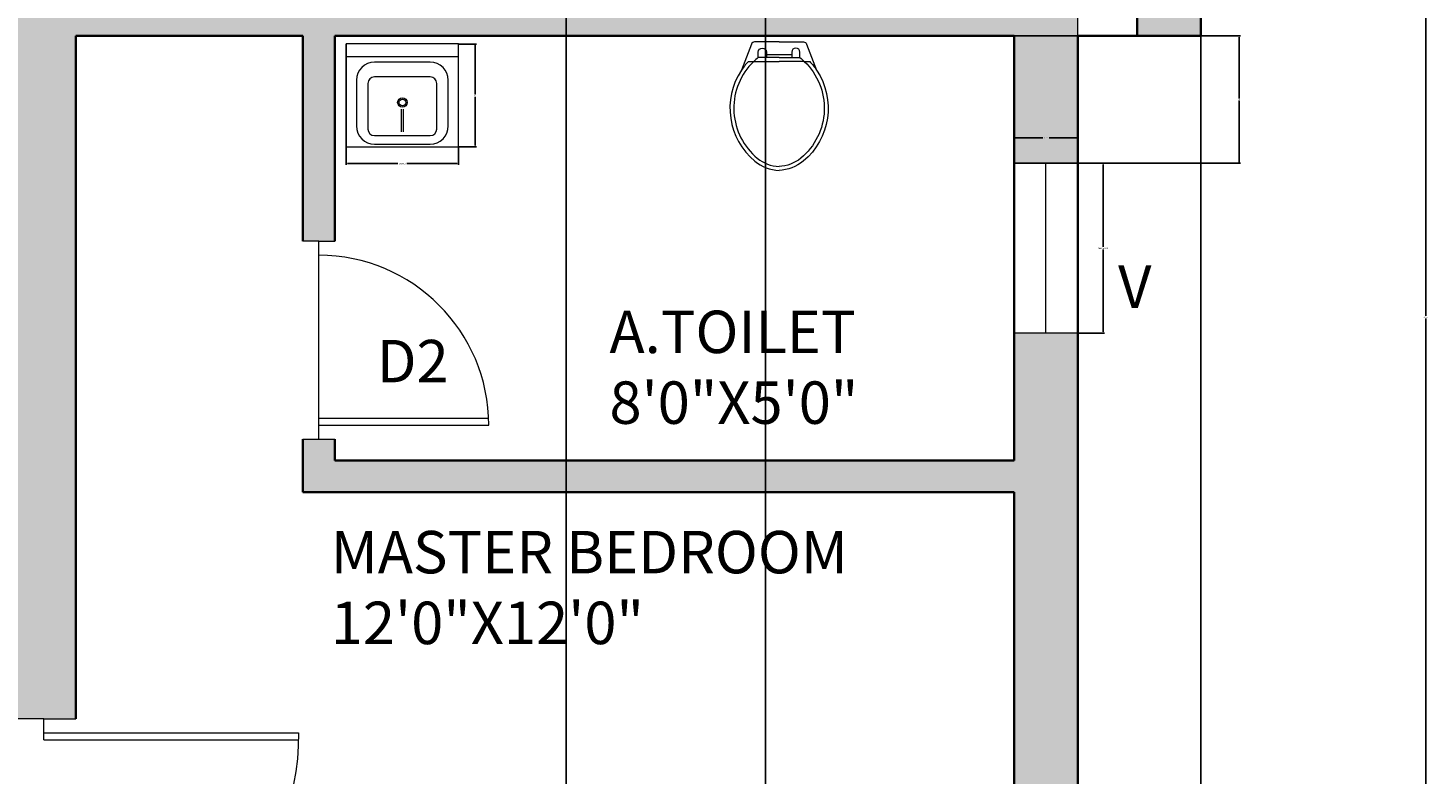
# Model space of a CAD drawing. Units: inches. Extents: x 5 to 421, y -617 to 43.
# Tile 9 of 15: x 223 to 421, y -351 to -246. Entities that reach past the tile are written whole.
import ezdxf

# ---------------------------------------------------------------- set-up
doc = ezdxf.new("R2010")
doc.units = ezdxf.units.IN
doc.header["$MEASUREMENT"] = 0
for name, color, linetype, lineweight in [('A-ANNO-DIMS', 2, 'Continuous', 18), ('A-ANNO-TEXT', 7, 'Continuous', 18), ('A-AREA-IDEN', 7, 'Continuous', 25), ('A-DOOR', 4, 'Continuous', 20), ('A-FLOR-FIXT', 9, 'Continuous', 18), ('A-GLAZ', 4, 'Continuous', 18), ('A-WALL', 7, 'Continuous', 35), ('WC-Detail_dwgmodels.com', 251, 'Continuous', 13), ('WC-Outline_dwgmodels.com', 250, 'Continuous', 18)]:
    doc.layers.add(name, color=color, linetype=linetype, lineweight=lineweight)
doc.layers.add('A-WALL-PATT', color=251, linetype='Continuous', lineweight=13, true_color=0x636466)
doc.styles.get("Standard").update_dxf_attribs({"font": 'arial.ttf'})
doc.dimstyles.get("Standard").update_dxf_attribs({"dimtxt": 0.18, "dimasz": 0.18, "dimexe": 0.18, "dimexo": 0.0625, "dimgap": 0.09, "dimtad": 0, "dimtih": 1, "dimtoh": 1, "dimdec": 0, "dimzin": 0, "dimdsep": 46, "dimlunit": 3, "dimtxsty": 'Standard', "dimcen": 0.09, "dimadec": 0, "dimazin": 0, "dimtfac": 1, "dimtdec": 0, "dimtofl": 0, "dimtmove": 0, "dimatfit": 3, "dimfxl": 1, "dimtolj": 1, "dimtzin": 0, "dimarcsym": 0})

# ---------------------------------------------------------------- blocks, each defined once
blk = doc.blocks.new('М14 600х655')
for p, q in [((-655, 600), (-655, 0)), ((-655, 600), (-655, 0)), ((-655, 0), (-655, 600)), ((0, 600), (-655, 600)), ((0, 0), (0, 600)), ((0, 525), (-655, 525)), ((-165.1, 494.1), (-489.9, 494.1)), ((-595.8, 388.1), (-595.8, 121.3)), ((-528.4, 370.1), (-528.4, 103.3)), ((-165.4, 408.4), (-490.2, 408.4)), ((-127.2, 103.3), (-127.2, 370.1)), ((-59.2, 121.3), (-59.2, 388.1)), ((-333.5, 87.1), (-333.5, 219.6)), ((-321.5, 87.1), (-321.5, 219.6)), ((-655, 0), (-655, 0)), ((-655, 0), (-655, 0)), ((-655, 0), (0, 0)), ((-655, 0), (0, 0)), ((-490.2, 65.1), (-165.4, 65.1)), ((-489.9, 15.4), (-165.1, 15.4))]:
    blk.add_line(p, q)
for radius in [27.6, 19.3]:
    blk.add_circle((-327.5, 258.9), radius)
for centre, radius, start, end in [((-489.9, 388.1), 105.9, 90, 180), ((-165.1, 388.1), 105.9, 0, 90), ((-490.2, 370.1), 38.2, 90, 180), ((-165.4, 370.1), 38.2, 0, 90), ((-489.9, 121.3), 105.9, 180, 270), ((-490.2, 103.3), 38.2, 180, 270), ((-165.4, 103.3), 38.2, 270, 0), ((-165.1, 121.3), 105.9, 270, 0)]:
    blk.add_arc(centre, radius, start, end)
blk = doc.blocks.new('VENT-24')
for p, q in [((0, 9), (24, 9)), ((0, 0), (0, 9)), ((24, 9), (24, 0)), ((0, 4.5), (24, 4.5)), ((24, 0), (0, 0))]:
    blk.add_line(p, q)
blk = doc.blocks.new('DOOR-SWING-36')
for p, q in [((35, 0), (35, 36)), ((36, 0), (36, 36))]:
    blk.add_line(p, q)
blk.add_arc((36, 0), 36, 90, 180)
blk = doc.blocks.new('DOOR-SWING-24')
for p, q in [((23, 0), (23, 24)), ((24, 0), (24, 24))]:
    blk.add_line(p, q)
blk.add_arc((24, 0), 24, 90, 180)
blk = doc.blocks.new('*D20')
at = {"layer": 'A-ANNO-DIMS', "color": 0, "lineweight": -2, "transparency": 16777216}
for p, q in [((371.09, -265.12), (374.81, -265.12)), ((374.63, -265.3), (374.63, -276.94)), ((374.63, -288.94), (374.63, -277.3)), ((371.09, -289.12), (374.81, -289.12))]:
    blk.add_line(p, q, dxfattribs=at)
at = {"layer": 'A-ANNO-DIMS', "color": 0, "transparency": 16777216}
for points in [[(374.6, -265.3), (374.66, -265.3), (374.63, -265.12)], [(374.6, -288.94), (374.66, -288.94), (374.63, -289.12)]]:
    blk.add_solid(points, dxfattribs=at)
at = {"layer": 'Defpoints', "color": 0, "transparency": 16777216}
for p in [(371.03, -265.12), (374.63, -265.12), (371.03, -289.12)]:
    blk.add_point(p, dxfattribs=at)
at = {"layer": 'A-ANNO-DIMS', "color": 0, "transparency": 16777216, "insert": (374.63, -277.12), "char_height": 0.18, "attachment_point": 5}
blk.add_mtext('\\A1;VENT 24 TYP.', dxfattribs=at)
blk = doc.blocks.new('*D21')
at = {"layer": 'A-ANNO-DIMS', "color": 0, "lineweight": -2, "transparency": 16777216}
for p, q in [((362.03, -265.06), (362.03, -261.34)), ((362.21, -261.52), (366.07, -261.52)), ((370.85, -261.52), (366.98, -261.52)), ((371.03, -265.06), (371.03, -261.34))]:
    blk.add_line(p, q, dxfattribs=at)
at = {"layer": 'A-ANNO-DIMS', "color": 0, "transparency": 16777216}
for points in [[(362.21, -261.49), (362.21, -261.55), (362.03, -261.52)], [(370.85, -261.49), (370.85, -261.55), (371.03, -261.52)]]:
    blk.add_solid(points, dxfattribs=at)
at = {"layer": 'Defpoints', "color": 0, "transparency": 16777216}
for p in [(362.03, -261.52), (362.03, -265.12), (371.03, -265.12)]:
    blk.add_point(p, dxfattribs=at)
at = {"layer": 'A-ANNO-DIMS', "color": 0, "transparency": 16777216, "insert": (366.53, -261.52), "char_height": 0.18, "attachment_point": 5}
blk.add_mtext('\\A1;9 TYP.', dxfattribs=at)
blk = doc.blocks.new('*D36')
at = {"layer": 'A-ANNO-DIMS', "color": 0, "lineweight": -2, "transparency": 16777216}
for p, q in [((267.65, -262.84), (267.65, -265.34)), ((283.51, -262.84), (283.51, -265.34)), ((267.83, -265.16), (274.95, -265.16)), ((283.33, -265.16), (276.2, -265.16))]:
    blk.add_line(p, q, dxfattribs=at)
at = {"layer": 'A-ANNO-DIMS', "color": 0, "transparency": 16777216}
for points in [[(267.83, -265.13), (267.83, -265.19), (267.65, -265.16)], [(283.33, -265.13), (283.33, -265.19), (283.51, -265.16)]]:
    blk.add_solid(points, dxfattribs=at)
at = {"layer": 'Defpoints', "color": 0, "transparency": 16777216}
for p in [(267.65, -262.78), (283.51, -262.78), (283.51, -265.16)]:
    blk.add_point(p, dxfattribs=at)
at = {"layer": 'A-ANNO-DIMS', "color": 0, "transparency": 16777216, "insert": (275.58, -265.16), "char_height": 0.18, "attachment_point": 5}
blk.add_mtext('\\A1;BASIN 16', dxfattribs=at)
blk = doc.blocks.new('*D37')
at = {"layer": 'A-ANNO-DIMS', "color": 0, "lineweight": -2, "transparency": 16777216}
for p, q in [((283.57, -248.26), (286.06, -248.26)), ((285.88, -248.44), (285.88, -255.34)), ((285.88, -262.6), (285.88, -255.7)), ((283.57, -262.78), (286.06, -262.78))]:
    blk.add_line(p, q, dxfattribs=at)
at = {"layer": 'A-ANNO-DIMS', "color": 0, "transparency": 16777216}
for points in [[(285.85, -248.44), (285.91, -248.44), (285.88, -248.26)], [(285.85, -262.6), (285.91, -262.6), (285.88, -262.78)]]:
    blk.add_solid(points, dxfattribs=at)
at = {"layer": 'Defpoints', "color": 0, "transparency": 16777216}
for p in [(283.51, -248.26), (285.88, -248.26), (283.51, -262.78)]:
    blk.add_point(p, dxfattribs=at)
at = {"layer": 'A-ANNO-DIMS', "color": 0, "transparency": 16777216, "insert": (285.88, -255.52), "char_height": 0.18, "attachment_point": 5}
blk.add_mtext('\\A1;15', dxfattribs=at)
blk = doc.blocks.new('*D55')
at = {"layer": 'A-ANNO-DIMS', "color": 0, "lineweight": -2, "transparency": 16777216}
for p, q in [((370.48, 10.88), (420.4, 10.88)), ((420.22, 10.7), (420.22, -286.69)), ((420.22, -584.44), (420.22, -287.05)), ((169.48, -584.62), (420.4, -584.62))]:
    blk.add_line(p, q, dxfattribs=at)
at = {"layer": 'A-ANNO-DIMS', "color": 0, "transparency": 16777216}
for points in [[(420.19, 10.7), (420.25, 10.7), (420.22, 10.88)], [(420.19, -584.44), (420.25, -584.44), (420.22, -584.62)]]:
    blk.add_solid(points, dxfattribs=at)
at = {"layer": 'Defpoints', "color": 0, "transparency": 16777216}
for p in [(370.42, 10.88), (169.42, -584.62), (420.22, -584.62)]:
    blk.add_point(p, dxfattribs=at)
at = {"layer": 'A-ANNO-DIMS', "color": 0, "transparency": 16777216, "insert": (420.22, -286.87), "char_height": 0.18, "attachment_point": 5}
blk.add_mtext('\\A1;595.5', dxfattribs=at)
blk = doc.blocks.new('*D65')
at = {"layer": 'A-ANNO-DIMS', "color": 0, "lineweight": -2, "transparency": 16777216}
for p, q in [((362.09, -247.12), (394.01, -247.12)), ((393.83, -247.3), (393.83, -255.94)), ((393.83, -264.94), (393.83, -256.3)), ((362.09, -265.12), (394.01, -265.12))]:
    blk.add_line(p, q, dxfattribs=at)
at = {"layer": 'A-ANNO-DIMS', "color": 0, "transparency": 16777216}
for points in [[(393.8, -247.3), (393.86, -247.3), (393.83, -247.12)], [(393.8, -264.94), (393.86, -264.94), (393.83, -265.12)]]:
    blk.add_solid(points, dxfattribs=at)
at = {"layer": 'Defpoints', "color": 0, "transparency": 16777216}
for p in [(362.03, -247.12), (362.03, -265.12), (393.83, -265.12)]:
    blk.add_point(p, dxfattribs=at)
at = {"layer": 'A-ANNO-DIMS', "color": 0, "transparency": 16777216, "insert": (393.83, -256.12), "char_height": 0.18, "attachment_point": 5}
blk.add_mtext('\\A1;18', dxfattribs=at)
blk = doc.blocks.new('*D69')
at = {"layer": 'A-ANNO-DIMS', "color": 0, "lineweight": -2, "transparency": 16777216}
for p, q in [((298.73, -207.41), (298.73, -616.6)), ((326.92, -207.41), (326.92, -616.6)), ((298.91, -616.42), (312.43, -616.42)), ((326.74, -616.42), (313.22, -616.42))]:
    blk.add_line(p, q, dxfattribs=at)
at = {"layer": 'A-ANNO-DIMS', "color": 0, "transparency": 16777216}
for points in [[(298.91, -616.39), (298.91, -616.45), (298.73, -616.42)], [(326.74, -616.39), (326.74, -616.45), (326.92, -616.42)]]:
    blk.add_solid(points, dxfattribs=at)
at = {"layer": 'Defpoints', "color": 0, "transparency": 16777216}
for p in [(298.73, -207.35), (326.92, -207.35), (326.92, -616.42)]:
    blk.add_point(p, dxfattribs=at)
at = {"layer": 'A-ANNO-DIMS', "color": 0, "transparency": 16777216, "insert": (312.82, -616.42), "char_height": 0.18, "attachment_point": 5}
blk.add_mtext('\\A1;28.19', dxfattribs=at)
blk = doc.blocks.new('*D73')
at = {"layer": 'A-ANNO-DIMS', "color": 0, "lineweight": -2, "transparency": 16777216}
for p, q in [((371.03, -247.18), (371.03, -616.6)), ((388.42, -247.18), (388.42, -616.6)), ((371.21, -616.42), (379.27, -616.42)), ((388.24, -616.42), (380.18, -616.42))]:
    blk.add_line(p, q, dxfattribs=at)
at = {"layer": 'A-ANNO-DIMS', "color": 0, "transparency": 16777216}
for points in [[(371.21, -616.39), (371.21, -616.45), (371.03, -616.42)], [(388.24, -616.39), (388.24, -616.45), (388.42, -616.42)]]:
    blk.add_solid(points, dxfattribs=at)
at = {"layer": 'Defpoints', "color": 0, "transparency": 16777216}
for p in [(371.03, -247.12), (388.42, -247.12), (388.42, -616.42)]:
    blk.add_point(p, dxfattribs=at)
at = {"layer": 'A-ANNO-DIMS', "color": 0, "transparency": 16777216, "insert": (379.72, -616.42), "char_height": 0.18, "attachment_point": 5}
blk.add_mtext('\\A1;17.393', dxfattribs=at)

msp = doc.modelspace()

# ---------------------------------------------------------------- hatches: boundary and pattern name
at = {"layer": 'A-WALL-PATT'}
h = msp.add_hatch(color=256, dxfattribs=at)
h.dxf.hatch_style = 1
h.paths.add_polyline_path([(46.4196, -88.1188), (37.4196, -88.1188), (37.4196, -166.6119), (46.4196, -166.6119), (46.4196, -122.6188), (135.4196, -122.6188), (135.4196, -120.3688), (135.4196, -118.1188), (46.4196, -118.1188)])
h.paths.add_polyline_path([(82.4196, 10.8812), (37.4196, 10.8812), (37.4196, -28.1188), (46.4196, -28.1188), (46.4196, 1.8812), (82.4196, 1.8812)])
h.paths.add_polyline_path([(215.5968, 10.8812), (142.4196, 10.8812), (142.4196, 1.8812), (178.4196, 1.8812), (178.4196, -118.1188), (175.4196, -118.1188), (175.4196, -122.6188), (182.9196, -122.6188), (182.9196, -80.6188), (211.9196, -80.6188), (211.9196, -78.3688), (211.9196, -76.1188), (182.9196, -76.1188), (182.9196, 1.8812), (215.5968, 1.8812)])
h.paths.add_polyline_path([(274.4196, 10.8812), (239.5968, 10.8812), (239.5968, 1.8812), (242.9196, 1.8812), (242.9196, -76.1188), (239.9196, -76.1188), (239.9196, -80.6188), (242.9196, -80.6188), (242.9196, -83.6188), (247.4196, -83.6188), (247.4196, 1.8812), (274.4196, 1.8812)])
h.paths.add_polyline_path([(370.4196, 10.8812), (334.4196, 10.8812), (334.4196, 1.8812), (361.4196, 1.8812), (361.4196, -28.1188), (370.4196, -28.1188)])
h.paths.add_polyline_path([(370.4196, -88.1188), (361.4196, -88.1188), (361.4196, -118.1188), (247.4196, -118.1188), (247.4196, -115.1188), (242.9196, -115.1188), (242.9196, -118.1188), (220.4196, -118.1188), (220.4196, -158.6188), (224.9196, -158.6188), (224.9196, -122.6188), (326.9196, -122.6188), (326.9196, -170.7662), (331.4196, -170.7662), (331.4196, -122.6188), (370.4196, -122.6188)])
h.paths.add_polyline_path([(388.4196, -122.6188), (388.4196, -118.1188), (379.4196, -118.1188), (379.4196, -122.6188), (379.4196, -154.8688), (388.4196, -154.8688)])
h.paths.add_polyline_path([(388.4196, -214.8688), (379.4196, -214.8688), (379.4196, -247.1188), (388.4196, -247.1188)])
h.paths.add_polyline_path([(371.0265, -242.6188), (331.4196, -242.6188), (331.4196, -239.6188), (326.9196, -239.6188), (326.9196, -242.6188), (224.9196, -242.6188), (224.9196, -206.6188), (220.4196, -206.6188), (220.4196, -343.6188), (224.9196, -343.6188), (229.4196, -343.6188), (229.4196, -247.1188), (261.5265, -247.1188), (261.5265, -276.1188), (263.7765, -276.1188), (266.0265, -276.1188), (266.0265, -247.1188), (362.0265, -247.1188), (362.0265, -265.1188), (371.0265, -265.1188), (371.0265, -247.1188)])
h.paths.add_polyline_path([(371.0265, -289.1188), (362.0265, -289.1188), (362.0265, -307.1188), (266.0265, -307.1188), (266.0265, -304.1188), (261.5265, -304.1188), (261.5265, -307.1188), (261.5265, -311.6188), (362.0265, -311.6188), (362.0265, -353.6188), (371.0265, -353.6188)])
h.paths.add_polyline_path([(371.0265, -413.6188), (362.0265, -413.6188), (362.0265, -455.6188), (325.7231, -455.6188), (325.7231, -464.6188), (361.4196, -464.6188), (371.0265, -464.6188)])
h.paths.add_polyline_path([(265.7231, -455.6188), (229.4196, -455.6188), (229.4196, -383.6188), (220.4196, -383.6188), (220.4196, -386.6188), (207.4649, -386.6188), (207.4649, -395.6188), (220.4196, -395.6188), (220.4196, -455.6188), (216.0568, -455.6188), (216.0568, -464.6188), (265.7231, -464.6188)])
h.paths.add_polyline_path([(169.4196, -386.6188), (137.9196, -386.6188), (137.9196, -395.6188), (160.4196, -395.6188), (160.4196, -424.2032), (169.4196, -424.2032)])
h.paths.add_polyline_path([(169.4196, -453.7423), (160.4196, -453.7423), (160.4196, -464.6188), (169.4196, -464.6188)])
h.paths.add_polyline_path([(46.4196, -575.6188), (37.4196, -575.6188), (37.4196, -584.6188), (46.4196, -584.6188)])
h.paths.add_polyline_path([(169.4196, -575.6188), (160.4196, -575.6188), (160.4196, -579.5504), (160.4196, -584.6188), (169.4196, -584.6188)])
h.paths.add_polyline_path([(46.4196, -226.6119), (37.4196, -226.6119), (37.4196, -292.8008), (46.4196, -292.8008)])
h.paths.add_polyline_path([(46.4196, -352.8008), (37.4196, -352.8008), (37.4196, -395.6188), (77.9196, -395.6188), (77.9196, -386.6188), (46.4196, -386.6188)])

# ---------------------------------------------------------------- linework, layer by layer
at = {"layer": 'A-DOOR'}
for p, q in [((263.7765, -276.1188), (261.5265, -276.1188)), ((263.7765, -278.1188), (263.7765, -276.1188)), ((263.7765, -276.1188), (266.0265, -276.1188)), ((263.7765, -302.1188), (263.7765, -278.1188)), ((263.7765, -304.1188), (263.7765, -302.1188)), ((261.5265, -304.1188), (266.0265, -304.1188)), ((224.9196, -343.6188), (220.4196, -343.6188)), ((224.9196, -346.6188), (224.9196, -343.6188)), ((224.9196, -343.6188), (229.4196, -343.6188))]:
    msp.add_line(p, q, dxfattribs=at)
at = {"layer": 'A-GLAZ'}
msp.add_line((371.0265, -247.1188), (371.0265, -242.6188), dxfattribs=at)
at = {"layer": 'A-WALL'}
for p, q in [((379.4196, -122.6188), (379.4196, -247.1188)), ((388.4196, -122.6188), (388.4196, -247.1188)), ((229.4196, -247.1188), (261.5265, -247.1188)), ((229.4196, -247.1188), (229.4196, -343.6188)), ((261.5265, -247.1188), (261.5265, -276.1188)), ((266.0265, -247.1188), (266.0265, -276.1188)), ((266.0265, -247.1188), (362.0265, -247.1188)), ((362.0265, -247.1188), (362.0265, -307.1188)), ((371.0265, -247.1188), (371.0265, -464.6188)), ((371.0265, -247.1188), (388.4196, -247.1188)), ((261.5265, -304.1188), (261.5265, -307.1188)), ((266.0265, -304.1188), (266.0265, -307.1188)), ((261.5265, -307.1188), (261.5265, -311.6188)), ((266.0265, -307.1188), (362.0265, -307.1188)), ((261.5265, -311.6188), (362.0265, -311.6188)), ((362.0265, -311.6188), (362.0265, -455.6188))]:
    msp.add_line(p, q, dxfattribs=at)
at = {"layer": 'WC-Detail_dwgmodels.com'}
for p, q in [((324.4761, -250.7164), (325.2377, -250.7164)), ((332.3822, -250.7164), (333.1438, -250.7164))]:
    msp.add_line(p, q, dxfattribs=at)
for points in [[(325.864, -250.1683), (325.864, -249.4062, -1), (327.0222, -249.4062), (327.0222, -249.8029)], [(331.7559, -250.1683), (331.7559, -249.4062, 1), (330.5977, -249.4062), (330.5977, -249.8029)], [(324.4761, -250.7164, 0.04093657), (323.4931, -251.9625, 0.16373228)], [(325.864, -250.1683, 0.02271164), (325.2377, -250.7164, 0.16261828)], [(328.81, -250.1683), (325.864, -250.1683, 0.02271164)], [(328.81, -250.1683), (331.7559, -250.1683, -0.47610764)], [(331.7559, -250.1683, -0.02271164), (332.3822, -250.7164, -0.16261828)], [(333.1438, -250.7164, -0.04093657), (334.1268, -251.9625, -0.16373228)]]:
    msp.add_lwpolyline(points, format="xyb", dxfattribs=at)
for points in [[(330.5977, -249.8029), (327.0222, -249.8029)], [(327.0222, -249.8029), (327.0222, -250.1683)], [(330.5977, -249.8029), (330.5977, -250.1683)]]:
    msp.add_lwpolyline(points, dxfattribs=at)
at = {"layer": 'WC-Outline_dwgmodels.com'}
for p in [(325.2377, -250.7164), (332.3822, -250.7164)]:
    msp.add_line(p, (328.81, -250.7164), dxfattribs=at)
for points in [[(328.81, -247.9674), (325.3427, -247.9674, 0.31031032), (324.9177, -248.2592), (323.4931, -251.9625, 0.20907131)], [(328.81, -247.9674), (332.2772, -247.9674, -0.31031032), (332.7022, -248.2592), (334.1268, -251.9625, -0.20907131)], [(324.8733, -251.0863, 0.43163885), (325.7424, -264.3982, 0.16261828), (328.81, -265.5817, 0.47087745)], [(325.2377, -250.7164, 0.01416454), (324.8733, -251.0863, 0.16261828)], [(332.3822, -250.7164, -0.44854579), (331.8775, -264.3982, -0.16261828), (328.81, -265.5817, -0.47087745)], [(323.4931, -251.9625, 0.38391851), (325.3967, -264.8165, 0.16373228), (328.81, -266.1249, 0.35973259)], [(334.1268, -251.9625, -0.38391851), (332.2232, -264.8165, -0.16373228), (328.81, -266.1249, -0.35973259)]]:
    msp.add_lwpolyline(points, format="xyb", dxfattribs=at)

# ---------------------------------------------------------------- block references
at = {"layer": 'A-DOOR', "rotation": 270.0000000000001}
msp.add_blockref('DOOR-SWING-24', (263.7765, -278.1188), dxfattribs=at)
at = {"layer": 'A-DOOR', "extrusion": (0, 0, -1), "zscale": -1, "rotation": 90.00000000000006}
msp.add_blockref('DOOR-SWING-36', (-224.9196, -381.6188), dxfattribs=at)
at = {"layer": 'A-FLOR-FIXT', "xscale": 0.0242100753764926, "yscale": 0.0242100753764926, "zscale": 0.0242100753764926}
msp.add_blockref('М14 600х655', (283.506, -262.7815), dxfattribs=at)
at = {"layer": 'A-GLAZ', "rotation": 89.99999999999991}
msp.add_blockref('VENT-24', (371.0265, -289.1188), dxfattribs=at)

# ---------------------------------------------------------------- texts
at = {"layer": 'A-ANNO-TEXT', "char_height": 6, "attachment_point": 1}
for s, insert in [('V', (376.7317, -279.5555)), ('D2', (271.9487, -290.0765))]:
    msp.add_mtext(s, dxfattribs=dict(at, insert=insert))
at = {"layer": 'A-AREA-IDEN', "char_height": 6, "attachment_point": 1}
for s, insert in [('A.TOILET\\P8\'0"X5\'0"', (304.8443, -285.9423)), ('MASTER BEDROOM\\P12\'0"X12\'0"', (265.4578, -317.0749))]:
    msp.add_mtext(s, dxfattribs=dict(at, insert=insert))

# ---------------------------------------------------------------- dimensions: what is measured, and where the dimension line sits
at = {"layer": 'A-ANNO-DIMS'}
for base, p1, p2, angle, override, picture, middle in [((420.2196, -584.6188), (370.4196, 10.8812), (169.4196, -584.6188), 90, {"dimdec": 1, "dimlfac": 1, "dimrnd": 0, "dimzin": 0, "dimdsep": 46, "dimlunit": 2}, '*D55', (420.2196, -286.8688)), ((393.8265, -265.1188), (362.0265, -247.1188), (362.0265, -265.1188), 270, {"dimdec": 0, "dimlfac": 1, "dimrnd": 0, "dimzin": 0, "dimdsep": 46, "dimlunit": 2}, '*D65', (393.8265, -256.1188)), ((285.8846, -248.2554), (283.506, -262.7815), (283.506, -248.2554), 90, {"dimdec": 0, "dimlfac": 1, "dimrnd": 0, "dimzin": 0, "dimdsep": 46, "dimlunit": 2}, '*D37', (285.8846, -255.5185))]:
    dim = msp.add_linear_dim(base=base, p1=p1, p2=p2, angle=angle, dimstyle='Standard', override=override, dxfattribs=at)
    dim.commit()
    dim.dimension.update_dxf_attribs({"geometry": picture, "text_midpoint": middle})
for base, p1, p2, override, picture, middle in [((326.9196, -616.4188), (298.7283, -207.3464), (326.9196, -207.3464), {"dimdec": 2, "dimlfac": 1, "dimrnd": 0, "dimzin": 0, "dimdsep": 46, "dimlunit": 2}, '*D69', (312.8239, -616.4188)), ((388.4196, -616.4188), (371.0265, -247.1188), (388.4196, -247.1188), {"dimdec": 3, "dimlfac": 1, "dimrnd": 0, "dimzin": 0, "dimdsep": 46, "dimlunit": 2}, '*D73', (379.7231, -616.4188))]:
    dim = msp.add_linear_dim(base=base, p1=p1, p2=p2, dimstyle='Standard', override=override, dxfattribs=at)
    dim.commit()
    dim.dimension.update_dxf_attribs({"geometry": picture, "text_midpoint": middle})
dim = msp.add_linear_dim(base=(283.506, -265.1601), p1=(267.6484, -262.7815), p2=(283.506, -262.7815), text='BASIN <>', dimstyle='Standard', override={"dimdec": 0, "dimlfac": 1, "dimrnd": 0, "dimzin": 0, "dimdsep": 46, "dimlunit": 2}, dxfattribs=at)
dim.commit()
dim.dimension.update_dxf_attribs({"geometry": '*D36', "text_midpoint": (275.5772, -265.1601)})
for base, p1, p2, angle, text, picture, middle in [((362.0265, -261.5188), (371.0265, -265.1188), (362.0265, -265.1188), 180, '<> TYP.', '*D21', (366.5265, -261.5188)), ((374.6265, -265.1188), (371.0265, -289.1188), (371.0265, -265.1188), 90, 'VENT <> TYP.', '*D20', (374.6265, -277.1188))]:
    dim = msp.add_linear_dim(base=base, p1=p1, p2=p2, angle=angle, text=text, dimstyle='Standard', override={"dimdec": 0, "dimlfac": 1, "dimrnd": 0, "dimzin": 0, "dimdsep": 46, "dimlunit": 2}, dxfattribs=at)
    dim.commit()
    dim.dimension.update_dxf_attribs({"geometry": picture, "text_midpoint": middle})

doc.saveas('drawing.dxf')
